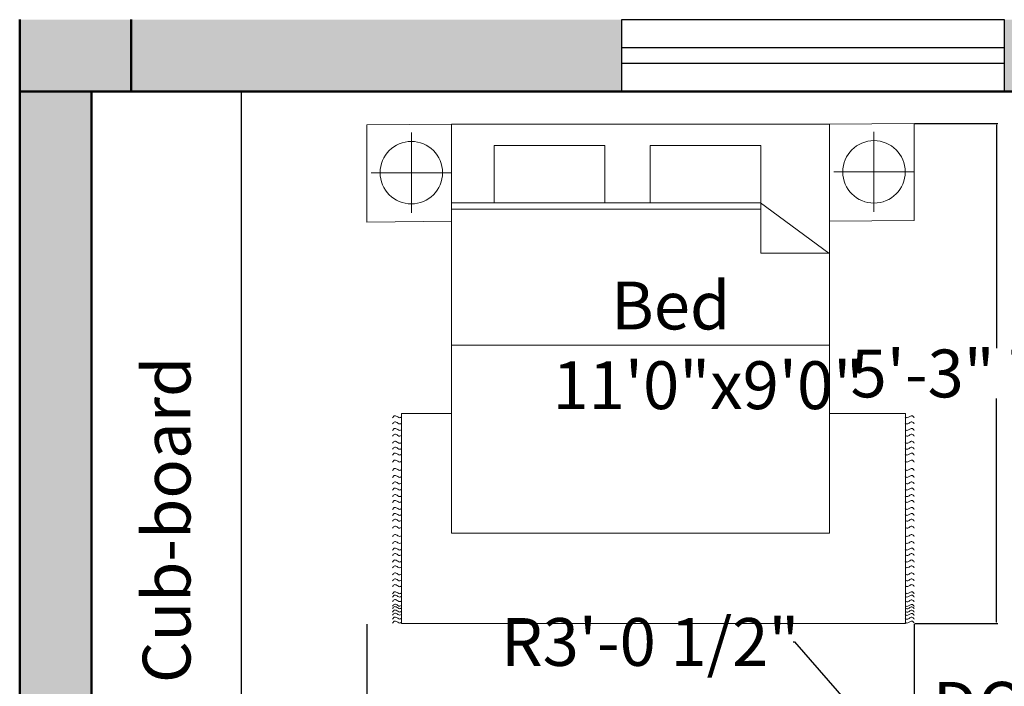
# Model space of a CAD drawing. Units: inches. Extents: x 1601 to 2080, y 5000 to 5589.
# Tile 9 of 11: x 1688 to 1812, y 5348 to 5431. Entities that reach past the tile are written whole.
import ezdxf

# ---------------------------------------------------------------- set-up
doc = ezdxf.new("R2010")
doc.units = ezdxf.units.IN
doc.header["$MEASUREMENT"] = 0
for name, color, linetype, lineweight in [('A-ANNO-DIMS', 2, 'Continuous', 18), ('A-ANNO-TEXT', 7, 'Continuous', 25), ('A-AREA-IDEN', 7, 'Continuous', 25), ('A-COLS', 7, 'Continuous', 50), ('A-COLS-PATT', 18, 'Continuous', 13), ('A-FLOR-CASE', 8, 'Continuous', 25), ('A-FLOR-PATT', 8, 'Continuous', 13), ('A-FURN', 8, 'Continuous', 18), ('A-GLAZ', 4, 'Continuous', 25), ('A-WALL', 7, 'Continuous', 50), ('A-WALL-PATT', 241, 'Continuous', 13)]:
    doc.layers.add(name, color=color, linetype=linetype, lineweight=lineweight)
doc.styles.get("Standard").update_dxf_attribs({"font": 'arial.ttf'})
doc.dimstyles.get("Standard").update_dxf_attribs({"dimtxt": 6, "dimasz": 0.18, "dimexe": 0.18, "dimexo": 0.0625, "dimgap": 0.09, "dimtad": 0, "dimtih": 1, "dimtoh": 1, "dimdec": 1, "dimzin": 0, "dimdsep": 46, "dimlunit": 3, "dimtxsty": 'Standard', "dimcen": 0.09, "dimadec": 0, "dimazin": 0, "dimtfac": 1, "dimtdec": 1, "dimtofl": 0, "dimtmove": 0, "dimatfit": 3, "dimfxl": 1, "dimtolj": 1, "dimtzin": 0, "dimarcsym": 0})

# ---------------------------------------------------------------- blocks, each defined once
blk = doc.blocks.new('BED-DOUBLE-ENSEMBLE')
for p, q in [((5.6, 61.61), (5.6, 51.56)), ((63.65, 61.72), (63.65, 51.66)), ((10.63, 56.59), (0.57, 56.59)), ((68.68, 56.69), (58.62, 56.69)), ((49.39, 52.82), (10.63, 52.82)), ((49.44, 52), (10.63, 52)), ((49.39, 52.82), (58, 46.47)), ((49.44, 52.82), (49.44, 46.47)), ((49.44, 46.47), (58, 46.47)), ((58.05, 34.96), (10.63, 34.96)), ((4.35, 0), (4.35, 26.37)), ((4.35, 26.37), (10.65, 26.37)), ((58.05, 26.37), (67.59, 26.37)), ((67.59, 26.37), (67.59, 0)), ((67.59, 0), (4.35, 0))]:
    blk.add_line(p, q)
for points in [[(0, 50.39), (10.63, 50.5), (10.63, 62.68), (0, 62.58)], [(58.05, 62.68), (58.05, 11.36), (10.63, 11.36), (10.63, 62.68)], [(58.05, 50.5), (68.68, 50.6), (68.68, 62.78), (58.05, 62.68)], [(29.88, 59.98), (29.88, 52.82), (15.98, 52.82), (15.98, 59.98)], [(49.44, 59.98), (49.44, 52.82), (35.55, 52.82), (35.55, 59.98)]]:
    blk.add_lwpolyline(points, close=True)
for centre in [(63.65, 56.69), (5.6, 56.59)]:
    blk.add_circle(centre, 3.92)
for points, knots in [([(3.23, 25.83), (3.32, 25.96), (3.52, 26.2), (3.86, 25.96), (4.14, 25.78), (4.29, 25.89), (4.35, 25.94)], [0, 0, 0, 0, 0.400747, 0.791423, 1.067667, 1.29709, 1.29709, 1.29709, 1.29709]), ([(68.71, 25.83), (68.61, 25.96), (68.42, 26.2), (68.08, 25.96), (67.8, 25.78), (67.65, 25.89), (67.58, 25.94)], [0, 0, 0, 0, 0.400747, 0.791423, 1.067667, 1.29709, 1.29709, 1.29709, 1.29709]), ([(3.23, 25.06), (3.32, 25.18), (3.52, 25.42), (3.86, 25.18), (4.14, 25), (4.29, 25.11), (4.35, 25.16)], [0, 0, 0, 0, 0.400747, 0.791423, 1.067667, 1.29709, 1.29709, 1.29709, 1.29709]), ([(68.71, 25.06), (68.61, 25.18), (68.42, 25.42), (68.08, 25.18), (67.8, 25), (67.65, 25.11), (67.58, 25.16)], [0, 0, 0, 0, 0.400747, 0.791423, 1.067667, 1.29709, 1.29709, 1.29709, 1.29709]), ([(3.23, 24.24), (3.32, 24.36), (3.52, 24.6), (3.86, 24.36), (4.14, 24.19), (4.29, 24.3), (4.35, 24.34)], [0, 0, 0, 0, 0.400747, 0.791423, 1.067667, 1.29709, 1.29709, 1.29709, 1.29709]), ([(3.23, 23.51), (3.32, 23.63), (3.52, 23.87), (3.86, 23.63), (4.14, 23.46), (4.29, 23.57), (4.35, 23.62)], [0, 0, 0, 0, 0.400747, 0.791423, 1.067667, 1.29709, 1.29709, 1.29709, 1.29709]), ([(68.71, 24.24), (68.61, 24.36), (68.42, 24.6), (68.08, 24.36), (67.8, 24.19), (67.65, 24.3), (67.58, 24.34)], [0, 0, 0, 0, 0.400747, 0.791423, 1.067667, 1.29709, 1.29709, 1.29709, 1.29709]), ([(68.71, 23.51), (68.61, 23.63), (68.42, 23.87), (68.08, 23.63), (67.8, 23.46), (67.65, 23.57), (67.58, 23.62)], [0, 0, 0, 0, 0.400747, 0.791423, 1.067667, 1.29709, 1.29709, 1.29709, 1.29709]), ([(3.23, 22.63), (3.32, 22.75), (3.52, 22.99), (3.86, 22.75), (4.14, 22.58), (4.29, 22.68), (4.35, 22.73)], [0, 0, 0, 0, 0.400747, 0.791423, 1.067667, 1.29709, 1.29709, 1.29709, 1.29709]), ([(68.71, 22.63), (68.61, 22.75), (68.42, 22.99), (68.08, 22.75), (67.8, 22.58), (67.65, 22.68), (67.58, 22.73)], [0, 0, 0, 0, 0.400747, 0.791423, 1.067667, 1.29709, 1.29709, 1.29709, 1.29709]), ([(3.23, 21.88), (3.32, 22), (3.52, 22.24), (3.86, 22), (4.14, 21.83), (4.29, 21.93), (4.35, 21.98)], [0, 0, 0, 0, 0.400747, 0.791423, 1.067667, 1.29709, 1.29709, 1.29709, 1.29709]), ([(3.23, 21.15), (3.32, 21.27), (3.52, 21.51), (3.86, 21.27), (4.14, 21.1), (4.29, 21.2), (4.35, 21.25)], [0, 0, 0, 0, 0.400747, 0.791423, 1.067667, 1.29709, 1.29709, 1.29709, 1.29709]), ([(68.71, 21.88), (68.61, 22), (68.42, 22.24), (68.08, 22), (67.8, 21.83), (67.65, 21.93), (67.58, 21.98)], [0, 0, 0, 0, 0.400747, 0.791423, 1.067667, 1.29709, 1.29709, 1.29709, 1.29709]), ([(68.71, 21.15), (68.61, 21.27), (68.42, 21.51), (68.08, 21.27), (67.8, 21.1), (67.65, 21.2), (67.58, 21.25)], [0, 0, 0, 0, 0.400747, 0.791423, 1.067667, 1.29709, 1.29709, 1.29709, 1.29709]), ([(3.23, 20.27), (3.32, 20.39), (3.52, 20.63), (3.86, 20.39), (4.14, 20.22), (4.29, 20.32), (4.35, 20.37)], [0, 0, 0, 0, 0.400747, 0.791423, 1.067667, 1.29709, 1.29709, 1.29709, 1.29709]), ([(68.71, 20.27), (68.61, 20.39), (68.42, 20.63), (68.08, 20.39), (67.8, 20.22), (67.65, 20.32), (67.58, 20.37)], [0, 0, 0, 0, 0.400747, 0.791423, 1.067667, 1.29709, 1.29709, 1.29709, 1.29709]), ([(3.23, 19.23), (3.32, 19.35), (3.52, 19.59), (3.86, 19.35), (4.14, 19.18), (4.29, 19.29), (4.35, 19.33)], [0, 0, 0, 0, 0.400747, 0.791423, 1.067667, 1.29709, 1.29709, 1.29709, 1.29709]), ([(3.23, 18.35), (3.32, 18.47), (3.52, 18.71), (3.86, 18.47), (4.14, 18.3), (4.29, 18.4), (4.35, 18.45)], [0, 0, 0, 0, 0.400747, 0.791423, 1.067667, 1.29709, 1.29709, 1.29709, 1.29709]), ([(68.71, 19.23), (68.61, 19.35), (68.42, 19.59), (68.08, 19.35), (67.8, 19.18), (67.65, 19.29), (67.58, 19.33)], [0, 0, 0, 0, 0.400747, 0.791423, 1.067667, 1.29709, 1.29709, 1.29709, 1.29709]), ([(68.71, 18.35), (68.61, 18.47), (68.42, 18.71), (68.08, 18.47), (67.8, 18.3), (67.65, 18.4), (67.58, 18.45)], [0, 0, 0, 0, 0.400747, 0.791423, 1.067667, 1.29709, 1.29709, 1.29709, 1.29709]), ([(3.23, 17.53), (3.32, 17.65), (3.52, 17.89), (3.86, 17.65), (4.14, 17.48), (4.29, 17.59), (4.35, 17.64)], [0, 0, 0, 0, 0.400747, 0.791423, 1.067667, 1.29709, 1.29709, 1.29709, 1.29709]), ([(68.71, 17.53), (68.61, 17.65), (68.42, 17.89), (68.08, 17.65), (67.8, 17.48), (67.65, 17.59), (67.58, 17.64)], [0, 0, 0, 0, 0.400747, 0.791423, 1.067667, 1.29709, 1.29709, 1.29709, 1.29709]), ([(3.23, 16.76), (3.32, 16.88), (3.52, 17.12), (3.86, 16.88), (4.14, 16.7), (4.29, 16.81), (4.35, 16.86)], [0, 0, 0, 0, 0.400747, 0.791423, 1.067667, 1.29709, 1.29709, 1.29709, 1.29709]), ([(3.23, 15.94), (3.32, 16.06), (3.52, 16.3), (3.86, 16.06), (4.14, 15.89), (4.29, 15.99), (4.35, 16.04)], [0, 0, 0, 0, 0.400747, 0.791423, 1.067667, 1.29709, 1.29709, 1.29709, 1.29709]), ([(68.71, 16.76), (68.61, 16.88), (68.42, 17.12), (68.08, 16.88), (67.8, 16.7), (67.65, 16.81), (67.58, 16.86)], [0, 0, 0, 0, 0.400747, 0.791423, 1.067667, 1.29709, 1.29709, 1.29709, 1.29709]), ([(68.71, 15.94), (68.61, 16.06), (68.42, 16.3), (68.08, 16.06), (67.8, 15.89), (67.65, 15.99), (67.58, 16.04)], [0, 0, 0, 0, 0.400747, 0.791423, 1.067667, 1.29709, 1.29709, 1.29709, 1.29709]), ([(3.23, 15.21), (3.32, 15.33), (3.52, 15.57), (3.86, 15.33), (4.14, 15.16), (4.29, 15.27), (4.35, 15.31)], [0, 0, 0, 0, 0.400747, 0.791423, 1.067667, 1.29709, 1.29709, 1.29709, 1.29709]), ([(68.71, 15.21), (68.61, 15.33), (68.42, 15.57), (68.08, 15.33), (67.8, 15.16), (67.65, 15.27), (67.58, 15.31)], [0, 0, 0, 0, 0.400747, 0.791423, 1.067667, 1.29709, 1.29709, 1.29709, 1.29709]), ([(3.23, 14.33), (3.32, 14.45), (3.52, 14.69), (3.86, 14.45), (4.14, 14.28), (4.29, 14.38), (4.35, 14.43)], [0, 0, 0, 0, 0.400747, 0.791423, 1.067667, 1.29709, 1.29709, 1.29709, 1.29709]), ([(3.23, 13.58), (3.32, 13.7), (3.52, 13.94), (3.86, 13.7), (4.14, 13.53), (4.29, 13.63), (4.35, 13.68)], [0, 0, 0, 0, 0.400747, 0.791423, 1.067667, 1.29709, 1.29709, 1.29709, 1.29709]), ([(68.71, 14.33), (68.61, 14.45), (68.42, 14.69), (68.08, 14.45), (67.8, 14.28), (67.65, 14.38), (67.58, 14.43)], [0, 0, 0, 0, 0.400747, 0.791423, 1.067667, 1.29709, 1.29709, 1.29709, 1.29709]), ([(68.71, 13.58), (68.61, 13.7), (68.42, 13.94), (68.08, 13.7), (67.8, 13.53), (67.65, 13.63), (67.58, 13.68)], [0, 0, 0, 0, 0.400747, 0.791423, 1.067667, 1.29709, 1.29709, 1.29709, 1.29709]), ([(3.23, 12.85), (3.32, 12.97), (3.52, 13.21), (3.86, 12.97), (4.14, 12.8), (4.29, 12.9), (4.35, 12.95)], [0, 0, 0, 0, 0.400747, 0.791423, 1.067667, 1.29709, 1.29709, 1.29709, 1.29709]), ([(68.71, 12.85), (68.61, 12.97), (68.42, 13.21), (68.08, 12.97), (67.8, 12.8), (67.65, 12.9), (67.58, 12.95)], [0, 0, 0, 0, 0.400747, 0.791423, 1.067667, 1.29709, 1.29709, 1.29709, 1.29709]), ([(3.23, 11.97), (3.32, 12.09), (3.52, 12.33), (3.86, 12.09), (4.14, 11.92), (4.29, 12.02), (4.35, 12.07)], [0, 0, 0, 0, 0.400747, 0.791423, 1.067667, 1.29709, 1.29709, 1.29709, 1.29709]), ([(3.23, 10.93), (3.32, 11.05), (3.52, 11.29), (3.86, 11.05), (4.14, 10.88), (4.29, 10.99), (4.35, 11.03)], [0, 0, 0, 0, 0.400747, 0.791423, 1.067667, 1.29709, 1.29709, 1.29709, 1.29709]), ([(68.71, 11.97), (68.61, 12.09), (68.42, 12.33), (68.08, 12.09), (67.8, 11.92), (67.65, 12.02), (67.58, 12.07)], [0, 0, 0, 0, 0.400747, 0.791423, 1.067667, 1.29709, 1.29709, 1.29709, 1.29709]), ([(68.71, 10.93), (68.61, 11.05), (68.42, 11.29), (68.08, 11.05), (67.8, 10.88), (67.65, 10.99), (67.58, 11.03)], [0, 0, 0, 0, 0.400747, 0.791423, 1.067667, 1.29709, 1.29709, 1.29709, 1.29709]), ([(3.23, 10.05), (3.32, 10.17), (3.52, 10.41), (3.86, 10.17), (4.14, 10), (4.29, 10.1), (4.35, 10.15)], [0, 0, 0, 0, 0.400747, 0.791423, 1.067667, 1.29709, 1.29709, 1.29709, 1.29709]), ([(68.71, 10.05), (68.61, 10.17), (68.42, 10.41), (68.08, 10.17), (67.8, 10), (67.65, 10.1), (67.58, 10.15)], [0, 0, 0, 0, 0.400747, 0.791423, 1.067667, 1.29709, 1.29709, 1.29709, 1.29709]), ([(3.23, 9.23), (3.32, 9.35), (3.52, 9.59), (3.86, 9.35), (4.14, 9.18), (4.29, 9.29), (4.35, 9.34)], [0, 0, 0, 0, 0.400747, 0.791423, 1.067667, 1.29709, 1.29709, 1.29709, 1.29709]), ([(3.23, 8.54), (3.32, 8.66), (3.52, 8.9), (3.86, 8.66), (4.14, 8.49), (4.29, 8.6), (4.35, 8.65)], [0, 0, 0, 0, 0.400747, 0.791423, 1.067667, 1.29709, 1.29709, 1.29709, 1.29709]), ([(68.71, 9.23), (68.61, 9.35), (68.42, 9.59), (68.08, 9.35), (67.8, 9.18), (67.65, 9.29), (67.58, 9.34)], [0, 0, 0, 0, 0.400747, 0.791423, 1.067667, 1.29709, 1.29709, 1.29709, 1.29709]), ([(68.71, 8.54), (68.61, 8.66), (68.42, 8.9), (68.08, 8.66), (67.8, 8.49), (67.65, 8.6), (67.58, 8.65)], [0, 0, 0, 0, 0.400747, 0.791423, 1.067667, 1.29709, 1.29709, 1.29709, 1.29709]), ([(3.23, 7.73), (3.32, 7.85), (3.52, 8.09), (3.86, 7.85), (4.14, 7.67), (4.29, 7.78), (4.35, 7.83)], [0, 0, 0, 0, 0.400747, 0.791423, 1.067667, 1.29709, 1.29709, 1.29709, 1.29709]), ([(68.71, 7.73), (68.61, 7.85), (68.42, 8.09), (68.08, 7.85), (67.8, 7.67), (67.65, 7.78), (67.58, 7.83)], [0, 0, 0, 0, 0.400747, 0.791423, 1.067667, 1.29709, 1.29709, 1.29709, 1.29709]), ([(3.23, 7), (3.32, 7.12), (3.52, 7.36), (3.86, 7.12), (4.14, 6.95), (4.29, 7.05), (4.35, 7.1)], [0, 0, 0, 0, 0.400747, 0.791423, 1.067667, 1.29709, 1.29709, 1.29709, 1.29709]), ([(3.23, 6.12), (3.32, 6.24), (3.52, 6.48), (3.86, 6.24), (4.14, 6.06), (4.29, 6.17), (4.35, 6.22)], [0, 0, 0, 0, 0.400747, 0.791423, 1.067667, 1.29709, 1.29709, 1.29709, 1.29709]), ([(68.71, 7), (68.61, 7.12), (68.42, 7.36), (68.08, 7.12), (67.8, 6.95), (67.65, 7.05), (67.58, 7.1)], [0, 0, 0, 0, 0.400747, 0.791423, 1.067667, 1.29709, 1.29709, 1.29709, 1.29709]), ([(68.71, 6.12), (68.61, 6.24), (68.42, 6.48), (68.08, 6.24), (67.8, 6.06), (67.65, 6.17), (67.58, 6.22)], [0, 0, 0, 0, 0.400747, 0.791423, 1.067667, 1.29709, 1.29709, 1.29709, 1.29709]), ([(3.23, 5.36), (3.32, 5.49), (3.52, 5.72), (3.86, 5.49), (4.14, 5.31), (4.29, 5.42), (4.35, 5.47)], [0, 0, 0, 0, 0.400747, 0.791423, 1.067667, 1.29709, 1.29709, 1.29709, 1.29709]), ([(68.71, 5.36), (68.61, 5.49), (68.42, 5.72), (68.08, 5.49), (67.8, 5.31), (67.65, 5.42), (67.58, 5.47)], [0, 0, 0, 0, 0.400747, 0.791423, 1.067667, 1.29709, 1.29709, 1.29709, 1.29709]), ([(3.23, 4.64), (3.32, 4.76), (3.52, 5), (3.86, 4.76), (4.14, 4.58), (4.29, 4.69), (4.35, 4.74)], [0, 0, 0, 0, 0.400747, 0.791423, 1.067667, 1.29709, 1.29709, 1.29709, 1.29709]), ([(3.23, 3.75), (3.32, 3.88), (3.52, 4.11), (3.86, 3.88), (4.14, 3.7), (4.29, 3.81), (4.35, 3.86)], [0, 0, 0, 0, 0.400747, 0.791423, 1.067667, 1.29709, 1.29709, 1.29709, 1.29709]), ([(68.71, 4.64), (68.61, 4.76), (68.42, 5), (68.08, 4.76), (67.8, 4.59), (67.66, 4.69), (67.59, 4.73)], [0, 0, 0, 0, 0.400747, 0.791423, 1.067667, 1.283686, 1.283686, 1.283686, 1.283686]), ([(68.71, 3.75), (68.61, 3.88), (68.42, 4.11), (68.08, 3.88), (67.8, 3.7), (67.66, 3.8), (67.59, 3.85)], [0, 0, 0, 0, 0.400747, 0.791423, 1.067667, 1.283686, 1.283686, 1.283686, 1.283686]), ([(3.23, 3.32), (3.32, 3.45), (3.51, 3.7), (3.86, 3.44), (4.14, 3.27), (4.29, 3.38), (4.35, 3.43)], [0, 0, 0, 0, 0.407265, 0.802015, 1.07826, 1.307683, 1.307683, 1.307683, 1.307683]), ([(3.23, 2.76), (3.32, 2.88), (3.52, 3.12), (3.86, 2.88), (4.14, 2.71), (4.29, 2.81), (4.35, 2.86)], [0, 0, 0, 0, 0.400747, 0.791423, 1.067667, 1.29709, 1.29709, 1.29709, 1.29709]), ([(68.71, 3.32), (68.61, 3.45), (68.42, 3.69), (68.08, 3.45), (67.8, 3.27), (67.66, 3.38), (67.59, 3.42)], [0, 0, 0, 0, 0.402903, 0.794912, 1.071156, 1.287177, 1.287177, 1.287177, 1.287177]), ([(68.71, 2.73), (68.61, 2.85), (68.42, 3.09), (68.08, 2.85), (67.8, 2.68), (67.66, 2.78), (67.59, 2.82)], [0, 0, 0, 0, 0.400747, 0.791423, 1.067667, 1.283686, 1.283686, 1.283686, 1.283686]), ([(3.23, 2.18), (3.32, 2.31), (3.52, 2.54), (3.86, 2.31), (4.14, 2.13), (4.29, 2.24), (4.35, 2.29)], [0, 0, 0, 0, 0.400747, 0.791423, 1.067667, 1.29709, 1.29709, 1.29709, 1.29709]), ([(3.23, 1.88), (3.32, 2), (3.52, 2.24), (3.86, 2), (4.14, 1.82), (4.29, 1.93), (4.35, 1.98)], [0, 0, 0, 0, 0.400747, 0.791423, 1.067667, 1.29709, 1.29709, 1.29709, 1.29709]), ([(3.23, 1.46), (3.32, 1.58), (3.52, 1.82), (3.86, 1.58), (4.14, 1.4), (4.29, 1.51), (4.35, 1.56)], [0, 0, 0, 0, 0.400747, 0.791423, 1.067667, 1.29709, 1.29709, 1.29709, 1.29709]), ([(3.23, 1.06), (3.32, 1.18), (3.52, 1.42), (3.86, 1.18), (4.14, 1.01), (4.29, 1.11), (4.35, 1.16)], [0, 0, 0, 0, 0.400747, 0.791423, 1.067667, 1.29709, 1.29709, 1.29709, 1.29709]), ([(68.71, 1.43), (68.61, 1.55), (68.42, 1.79), (68.08, 1.55), (67.8, 1.38), (67.65, 1.48), (67.58, 1.53)], [0, 0, 0, 0, 0.400747, 0.791423, 1.067667, 1.29709, 1.29709, 1.29709, 1.29709]), ([(68.71, 1.03), (68.61, 1.15), (68.42, 1.39), (68.08, 1.15), (67.8, 0.98), (67.65, 1.09), (67.58, 1.13)], [0, 0, 0, 0, 0.400747, 0.791423, 1.067667, 1.29709, 1.29709, 1.29709, 1.29709]), ([(68.71, 2.16), (68.61, 2.28), (68.42, 2.52), (68.08, 2.28), (67.8, 2.11), (67.66, 2.21), (67.59, 2.25)], [0, 0, 0, 0, 0.400747, 0.791423, 1.067667, 1.283686, 1.283686, 1.283686, 1.283686]), ([(68.71, 1.85), (68.61, 1.97), (68.42, 2.21), (68.08, 1.97), (67.8, 1.8), (67.66, 1.9), (67.59, 1.94)], [0, 0, 0, 0, 0.400747, 0.791423, 1.067667, 1.283686, 1.283686, 1.283686, 1.283686]), ([(3.23, 0.57), (3.32, 0.7), (3.52, 0.93), (3.86, 0.7), (4.14, 0.52), (4.29, 0.63), (4.35, 0.68)], [0, 0, 0, 0, 0.400747, 0.791423, 1.067667, 1.29709, 1.29709, 1.29709, 1.29709]), ([(3.23, 0.07), (3.32, 0.19), (3.52, 0.43), (3.86, 0.19), (4.14, 0.02), (4.29, 0.13), (4.35, 0.18)], [0, 0, 0, 0, 0.400747, 0.791423, 1.067667, 1.29709, 1.29709, 1.29709, 1.29709]), ([(68.71, 0.55), (68.61, 0.67), (68.42, 0.91), (68.08, 0.67), (67.8, 0.49), (67.65, 0.6), (67.58, 0.65)], [0, 0, 0, 0, 0.400747, 0.791423, 1.067667, 1.29709, 1.29709, 1.29709, 1.29709]), ([(68.71, 0.07), (68.61, 0.19), (68.42, 0.43), (68.08, 0.19), (67.8, 0.02), (67.65, 0.13), (67.58, 0.18)], [0, 0, 0, 0, 0.400747, 0.791423, 1.067667, 1.29709, 1.29709, 1.29709, 1.29709])]:
    blk.add_open_spline(points, degree=3, knots=knots)
blk = doc.blocks.new('WINDOW-48IN')
for p, q in [((0, 0), (0, 9)), ((0, 9), (48, 9)), ((48, 9), (48, 0)), ((0, 5.5), (48, 5.5)), ((48, 3.5), (0, 3.5)), ((48, 0), (0, 0))]:
    blk.add_line(p, q)
blk = doc.blocks.new('*D17')
at = {"layer": 'A-ANNO-DIMS', "color": 0, "lineweight": -2, "transparency": 16777216}
for p, q in [((1731.95, 5355.35), (1731.95, 5344.92)), ((1800.66, 5355.35), (1800.66, 5344.92)), ((1732.13, 5345.1), (1800.48, 5345.1)), ((1800.66, 5345.1), (1800.84, 5345.1))]:
    blk.add_line(p, q, dxfattribs=at)
at = {"layer": 'A-ANNO-DIMS', "color": 0, "transparency": 16777216}
for points in [[(1732.13, 5345.13), (1732.13, 5345.07), (1731.95, 5345.1)], [(1800.48, 5345.13), (1800.48, 5345.07), (1800.66, 5345.1)]]:
    blk.add_solid(points, dxfattribs=at)
at = {"layer": 'Defpoints', "color": 0, "transparency": 16777216}
for p in [(1731.95, 5355.41), (1800.66, 5355.41), (1800.66, 5345.1)]:
    blk.add_point(p, dxfattribs=at)
at = {"layer": 'A-ANNO-DIMS', "color": 0, "transparency": 16777216, "insert": (1854.24, 5345.1), "char_height": 6, "attachment_point": 5}
blk.add_mtext('\\A1;DOUBLE BED 5\'-8 1/2" TYP.', dxfattribs=at)
blk = doc.blocks.new('*D18')
at = {"layer": 'A-ANNO-DIMS', "color": 0, "lineweight": -2, "transparency": 16777216}
for p, q in [((1800.72, 5418.19), (1811.15, 5418.19)), ((1810.97, 5418.01), (1810.97, 5389.96)), ((1810.97, 5355.59), (1810.97, 5383.65)), ((1800.72, 5355.41), (1811.15, 5355.41))]:
    blk.add_line(p, q, dxfattribs=at)
at = {"layer": 'A-ANNO-DIMS', "color": 0, "transparency": 16777216}
for points in [[(1810.94, 5418.01), (1811, 5418.01), (1810.97, 5418.19)], [(1810.94, 5355.59), (1811, 5355.59), (1810.97, 5355.41)]]:
    blk.add_solid(points, dxfattribs=at)
at = {"layer": 'Defpoints', "color": 0, "transparency": 16777216}
for p in [(1800.66, 5418.19), (1810.97, 5418.19), (1800.66, 5355.41)]:
    blk.add_point(p, dxfattribs=at)
at = {"layer": 'A-ANNO-DIMS', "color": 0, "transparency": 16777216, "insert": (1810.97, 5386.8), "char_height": 6, "attachment_point": 5}
blk.add_mtext('\\A1;5\'-3" TYP.', dxfattribs=at)
blk = doc.blocks.new('*D60')
at = {"layer": 'A-ANNO-DIMS', "color": 0, "lineweight": -2, "transparency": 16777216}
for p, q in [((1785.46, 5353.11), (1785.64, 5353.11)), ((1785.64, 5353.11), (1799.87, 5336.85)), ((1823.82, 5309.37), (1824, 5309.37)), ((1823.91, 5309.28), (1823.91, 5309.46))]:
    blk.add_line(p, q, dxfattribs=at)
at = {"layer": 'A-ANNO-DIMS', "color": 0, "transparency": 16777216}
blk.add_solid([(1799.89, 5336.86), (1799.85, 5336.83), (1799.99, 5336.71)], dxfattribs=at)
at = {"layer": 'Defpoints', "color": 0, "transparency": 16777216}
for p in [(1799.99, 5336.71), (1823.91, 5309.37)]:
    blk.add_point(p, dxfattribs=at)
at = {"layer": 'A-ANNO-DIMS', "color": 0, "transparency": 16777216, "insert": (1767.53, 5353.11), "char_height": 6, "attachment_point": 5}
blk.add_mtext('\\A1;R3\'-0 1/2"', dxfattribs=at)

msp = doc.modelspace()

# ---------------------------------------------------------------- hatches: boundary and pattern name
at = {"layer": 'A-COLS-PATT'}
h = msp.add_hatch(color=256, dxfattribs=at)
h.dxf.hatch_style = 1
h.paths.add_polyline_path([(1702.41, 5431.2), (1688.41, 5431.2), (1688.41, 5422.2), (1702.41, 5422.2)])
h.paths.add_polyline_path([(1836.17, 5431.2), (1822.17, 5431.2), (1822.17, 5422.2), (1836.17, 5422.2)])
h.paths.add_polyline_path([(1962.91, 5431.2), (1948.91, 5431.2), (1948.91, 5422.2), (1962.91, 5422.2)])
h.paths.add_polyline_path([(1697.41, 5314.2), (1688.41, 5314.2), (1688.41, 5300.2), (1697.41, 5300.2)])
h.paths.add_polyline_path([(1833.91, 5314.2), (1824.91, 5314.2), (1824.91, 5300.2), (1833.91, 5300.2)])
h.paths.add_polyline_path([(1962.91, 5314.2), (1953.91, 5314.2), (1953.91, 5300.2), (1962.91, 5300.2)])
h.paths.add_polyline_path([(1697.41, 5209.2), (1688.41, 5209.2), (1688.41, 5195.2), (1697.41, 5195.2)])
h.paths.add_polyline_path([(1833.91, 5209.2), (1824.91, 5209.2), (1824.91, 5195.2), (1833.91, 5195.2)])
h.paths.add_polyline_path([(1962.91, 5209.2), (1953.91, 5209.2), (1953.91, 5195.2), (1962.91, 5195.2)])
h.paths.add_polyline_path([(1697.41, 5083.7), (1688.41, 5083.7), (1688.41, 5069.7), (1697.41, 5069.7)])
h.paths.add_polyline_path([(1833.91, 5078.7), (1819.91, 5078.7), (1819.91, 5069.7), (1833.91, 5069.7)])
h.paths.add_polyline_path([(1962.91, 5078.7), (1948.91, 5078.7), (1948.91, 5069.7), (1962.91, 5069.7)])
at = {"layer": 'A-FLOR-PATT'}
h = msp.add_hatch(dxfattribs=at)
h.set_pattern_fill('ANGLE', color=256, scale=40)
h.set_pattern_definition([(0, (0, 0), (0, 11), [8, -3]), (90, (0, 0), (-11, 7e-16), [8, -3])])
h.paths.add_polyline_path([(2022.91, 5509.2), (1941.91, 5509.2), (1911.91, 5509.2), (1864.41, 5509.2), (1864.41, 5489.7), (1868.54, 5489.7, -0.022155), (1868.52, 5490.01, -1), (1875.53, 5490.01, -0.956651), (1868.54, 5489.7), (1864.41, 5489.7), (1864.41, 5470.2), (1794.41, 5470.2), (1794.41, 5431.2), (1811.95, 5431.2), (1911.91, 5431.2), (1941.91, 5431.2), (1942.91, 5431.2), (1945.91, 5431.2), (1948.91, 5431.2), (1962.91, 5431.2), (1962.91, 5415.29), (1962.91, 5385.29), (1962.91, 5384.29), (1962.91, 5381.29), (1962.91, 5333.29), (1962.91, 5069.7), (2022.91, 5069.7)])
h.paths.add_polyline_path([(2000.28, 5267.55), (2000.28, 5367.64), (1987.91, 5367.64), (1987.91, 5267.55)], flags=24)
h.paths.add_polyline_path([(1879.42, 5455.52), (1969.04, 5455.52), (1969.04, 5467.88), (1879.42, 5467.88)], flags=24)
at = {"layer": 'A-WALL-PATT'}
h = msp.add_hatch(color=256, dxfattribs=at)
h.dxf.hatch_style = 1
h.paths.add_polyline_path([(1763.95, 5431.2), (1702.41, 5431.2), (1702.41, 5422.2), (1763.95, 5422.2)])
h.paths.add_polyline_path([(1697.41, 5422.2), (1688.41, 5422.2), (1688.41, 5314.2), (1697.41, 5314.2)])
h.paths.add_polyline_path([(1740.41, 5314.2), (1697.41, 5314.2), (1697.41, 5309.7), (1740.41, 5309.7)], flags=17)
h.paths.add_polyline_path([(1822.17, 5431.2), (1811.95, 5431.2), (1811.95, 5422.2), (1822.17, 5422.2)])
h.paths.add_polyline_path([(1845.52, 5431.2), (1836.17, 5431.2), (1836.17, 5422.2), (1845.52, 5422.2)])
h.paths.add_polyline_path([(1910.91, 5431.2), (1881.52, 5431.2), (1881.52, 5422.2), (1910.91, 5422.2)])
h.paths.add_polyline_path([(1948.91, 5431.2), (1945.91, 5431.2), (1942.91, 5431.2), (1942.91, 5422.2), (1948.91, 5422.2)])
h.paths.add_polyline_path([(1962.91, 5422.2), (1953.91, 5422.2), (1953.91, 5416.29), (1962.91, 5416.29)])
h.paths.add_polyline_path([(1962.91, 5384.29), (1953.91, 5384.29), (1953.91, 5381.29), (1962.91, 5381.29)])
h.paths.add_polyline_path([(1962.91, 5333.29), (1953.91, 5333.29), (1953.91, 5314.2), (1962.91, 5314.2)])
h.paths.add_polyline_path([(1962.91, 5300.2), (1953.91, 5300.2), (1953.91, 5236.2), (1875.91, 5236.2), (1875.91, 5230.7), (1881.91, 5230.7), (1881.91, 5231.7), (1953.91, 5231.7), (1953.91, 5219.2), (1962.91, 5219.2)])
h.paths.add_polyline_path([(1962.91, 5185.2), (1953.91, 5185.2), (1953.91, 5183.7), (1881.91, 5183.7), (1881.91, 5184.7), (1875.91, 5184.7), (1875.91, 5183.7), (1875.91, 5179.2), (1953.91, 5179.2), (1953.91, 5172.6), (1962.91, 5172.6)])
h.paths.add_polyline_path([(1962.91, 5136.6), (1953.91, 5136.6), (1953.91, 5078.7), (1962.91, 5078.7)])
h.paths.add_polyline_path([(1948.91, 5078.7), (1833.91, 5078.7), (1833.91, 5069.7), (1948.91, 5069.7)])
h.paths.add_polyline_path([(1833.91, 5195.2), (1829.41, 5195.2), (1829.41, 5078.7), (1833.91, 5078.7)])
h.paths.add_polyline_path([(1819.91, 5078.7), (1813.58, 5078.7), (1813.58, 5069.7), (1819.91, 5069.7)])
h.paths.add_polyline_path([(1765.58, 5078.7), (1697.41, 5078.7), (1697.41, 5069.7), (1765.58, 5069.7)])
h.paths.add_polyline_path([(1697.41, 5195.2), (1688.41, 5195.2), (1688.41, 5083.7), (1697.41, 5083.7)])
h.paths.add_polyline_path([(1740.41, 5209.2), (1697.41, 5209.2), (1697.41, 5204.7), (1740.41, 5204.7)], flags=17)
h.paths.add_polyline_path([(1787.91, 5209.2), (1779.91, 5209.2), (1779.91, 5309.7), (1787.91, 5309.7), (1787.91, 5314.2), (1772.41, 5314.2), (1772.41, 5309.7), (1775.41, 5309.7), (1775.41, 5261.7), (1697.41, 5261.7), (1697.41, 5273.07), (1688.41, 5273.07), (1688.41, 5242.37), (1697.41, 5242.37), (1697.41, 5257.2), (1775.41, 5257.2), (1775.41, 5209.2), (1772.41, 5209.2), (1772.41, 5204.7), (1775.41, 5204.7), (1787.91, 5204.7)])
h.paths.add_polyline_path([(1697.41, 5218.37), (1688.41, 5218.37), (1688.41, 5209.2), (1697.41, 5209.2)], flags=17)
h.paths.add_polyline_path([(1833.91, 5422.2), (1829.41, 5422.2), (1829.41, 5314.2), (1833.91, 5314.2)])
h.paths.add_polyline_path([(1697.41, 5300.2), (1688.41, 5300.2), (1688.41, 5297.07), (1697.41, 5297.07)], flags=17)

# ---------------------------------------------------------------- linework, layer by layer
at = {"layer": 'A-COLS'}
msp.add_line((1702.41, 5431.2), (1702.41, 5422.2), dxfattribs=at)
at = {"layer": 'A-FLOR-CASE'}
msp.add_line((1716.19, 5422.2), (1716.19, 5314.2), dxfattribs=at)
at = {"layer": 'A-WALL'}
for p, q in [((1688.41, 5431.2), (1688.41, 5069.7)), ((1688.41, 5422.2), (1910.91, 5422.2)), ((1697.41, 5422.2), (1697.41, 5261.7))]:
    msp.add_line(p, q, dxfattribs=at)

# ---------------------------------------------------------------- block references
at = {"layer": 'A-FURN'}
msp.add_blockref('BED-DOUBLE-ENSEMBLE', (1731.95, 5355.41), dxfattribs=at)
at = {"layer": 'A-GLAZ'}
msp.add_blockref('WINDOW-48IN', (1763.95, 5422.2), dxfattribs=at)

# ---------------------------------------------------------------- texts
at = {"layer": 'A-ANNO-TEXT', "insert": (1703.84, 5347.95), "char_height": 6, "attachment_point": 1, "rotation": 90}
msp.add_mtext_dynamic_manual_height_columns('Cub-board', width=45.9316, gutter_width=30, heights=[0], dxfattribs=at)
at = {"layer": 'A-AREA-IDEN', "insert": (1755.26, 5398.33), "char_height": 6, "attachment_point": 1}
msp.add_mtext_dynamic_manual_height_columns('    Bed\\P11\'0"x9\'0"', width=45.8143, gutter_width=30, heights=[0], dxfattribs=at)

# ---------------------------------------------------------------- dimensions: what is measured, and where the dimension line sits
at = {"layer": 'A-ANNO-DIMS'}
dim = msp.add_linear_dim(base=(1810.97, 5418.19), p1=(1800.66, 5355.41), p2=(1800.66, 5418.19), angle=90, text='<> TYP.', dimstyle='Standard', override={"dimdec": 1, "dimlfac": 1, "dimrnd": 0, "dimzin": 1, "dimdsep": 46, "dimlunit": 4, "dimfrac": 2}, dxfattribs=at)
dim.commit()
dim.dimension.update_dxf_attribs({"geometry": '*D18', "text_midpoint": (1810.97, 5386.8)})
dim = msp.add_linear_dim(base=(1800.66, 5345.1), p1=(1731.95, 5355.41), p2=(1800.66, 5355.41), text='DOUBLE BED <> TYP.', dimstyle='Standard', override={"dimdec": 1, "dimlfac": 1, "dimrnd": 0, "dimzin": 1, "dimdsep": 46, "dimlunit": 4, "dimfrac": 2}, dxfattribs=at)
dim.commit()
dim.dimension.update_dxf_attribs({"geometry": '*D17', "text_midpoint": (1854.24, 5345.1)})
dim = msp.add_radius_dim(center=(1823.91, 5309.37), mpoint=(1799.99, 5336.71), dimstyle='Standard', override={"dimdec": 1, "dimlfac": 1, "dimrnd": 0, "dimzin": 1, "dimdsep": 46, "dimlunit": 4, "dimfrac": 2}, dxfattribs=at)
dim.commit()
dim.dimension.update_dxf_attribs({"geometry": '*D60', "text_midpoint": (1767.53, 5353.11), "dimtype": 164})

doc.saveas('drawing.dxf')
